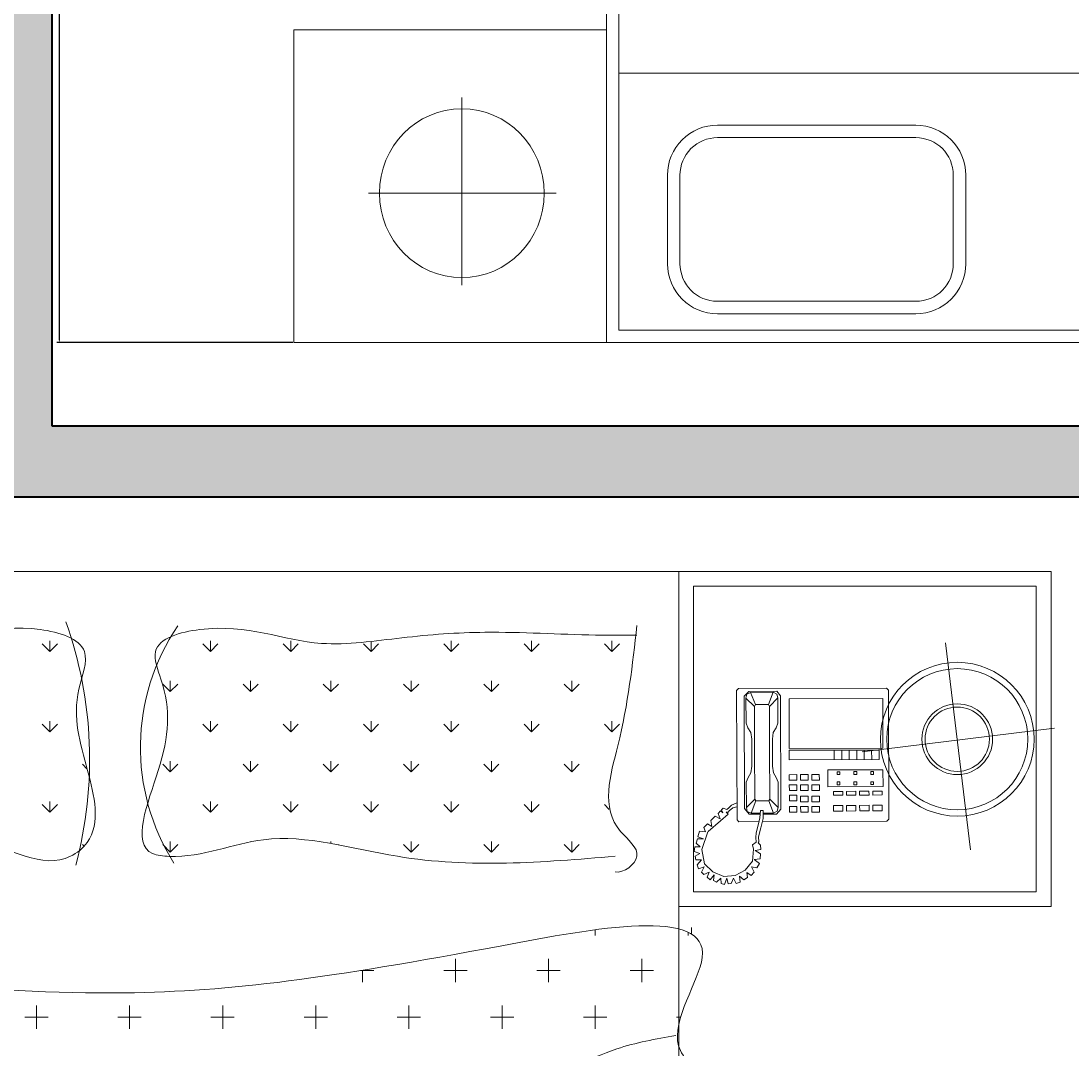
# Model space of a CAD drawing. Units: inches. Extents: x 2330 to 3943, y 1763 to 3461.
# Tile 20 of 40: x 3157 to 3231, y 2662 to 2734. Entities that reach past the tile are written whole.
import ezdxf

# ---------------------------------------------------------------- set-up
doc = ezdxf.new("R2010")
doc.units = ezdxf.units.IN
for name, color, linetype, lineweight in [('A-ANNO-DIMS', 2, 'Continuous', 18), ('A-FURN', 8, 'Continuous', 13), ('A-WALL', 7, 'Continuous', 40), ('A-WALL-PATT', 252, 'Continuous', 13)]:
    doc.layers.add(name, color=color, linetype=linetype, lineweight=lineweight)
doc.styles.get("Standard").update_dxf_attribs({"font": 'arial.ttf'})
doc.dimstyles.get("Standard").update_dxf_attribs({"dimtxt": 0.18, "dimasz": 0.18, "dimexe": 0.18, "dimexo": 0.0625, "dimgap": 0.09, "dimtad": 0, "dimtih": 1, "dimtoh": 1, "dimdec": 4, "dimzin": 0, "dimdsep": 46, "dimtxsty": 'Standard', "dimcen": 0.09, "dimadec": 0, "dimazin": 0, "dimtfac": 1, "dimtdec": 4, "dimtofl": 0, "dimtmove": 0, "dimatfit": 3, "dimfxl": 1, "dimtolj": 1, "dimtzin": 0, "dimarcsym": 0})

# ---------------------------------------------------------------- blocks, each defined once
blk = doc.blocks.new('A$C200C7901')
for p, q in [((0.5, 2.3334), (2, 2.3334)), ((2, 2.3334), (2.5, 2.3334)), ((2, 1.6055), (2, 2.3334)), ((2.5, 1.8834), (2.5, 2.3334)), ((1.3176, 2.1721), (1.3075, 2.1822)), ((1.3176, 2.1721), (1.3075, 2.1822)), ((1.206, 2.0681), (1.1997, 2.0744)), ((1.206, 2.0681), (1.1997, 2.0744)), ((1.2019, 1.9645), (1.1997, 1.9666)), ((1.2019, 1.9645), (1.1997, 1.9666)), ((2, 1.8834), (2.5, 1.8834)), ((2.0129, 1.8445), (2.0129, 1.849)), ((2.0129, 1.8445), (2.0129, 1.849)), ((2.0171, 1.8467), (2.0171, 1.8556)), ((2.0171, 1.8467), (2.0171, 1.8556)), ((1.1379, 1.7195), (1.1379, 1.7508)), ((1.1222, 1.7352), (1.1535, 1.7352)), ((1.9972, 1.7352), (2.0027, 1.7352)), ((1.9972, 1.7352), (2.0027, 1.7352)), ((2, 1.6963), (2, 1.7248)), ((2, 1.6963), (2, 1.7248))]:
    blk.add_line(p, q)
at = {"linetype": 'ByBlock'}
for p, q in [((2.02, 2.3134), (2.48, 2.3134)), ((2.02, 1.9034), (2.02, 2.3134)), ((2.48, 1.9034), (2.48, 2.3134)), ((1.1559, 2.2259), (1.1458, 2.236)), ((1.1559, 2.2259), (1.1458, 2.236)), ((1.1559, 2.2259), (1.1559, 2.2402)), ((1.1559, 2.2259), (1.1559, 2.2402)), ((1.1559, 2.2259), (1.166, 2.236)), ((1.1559, 2.2259), (1.166, 2.236)), ((1.3714, 2.2259), (1.3613, 2.236)), ((1.3714, 2.2259), (1.3613, 2.236)), ((1.3714, 2.2259), (1.3714, 2.2402)), ((1.3714, 2.2259), (1.3714, 2.2402)), ((1.3714, 2.2259), (1.3815, 2.236)), ((1.3714, 2.2259), (1.3815, 2.236)), ((1.4792, 2.2259), (1.4691, 2.236)), ((1.4792, 2.2259), (1.4691, 2.236)), ((1.4792, 2.2259), (1.4792, 2.2402)), ((1.4792, 2.2259), (1.4792, 2.2402)), ((1.4792, 2.2259), (1.4893, 2.236)), ((1.4792, 2.2259), (1.4893, 2.236)), ((1.587, 2.2259), (1.5769, 2.236)), ((1.587, 2.2259), (1.5769, 2.236)), ((1.587, 2.2259), (1.587, 2.2393)), ((1.587, 2.2259), (1.587, 2.2393)), ((1.587, 2.2259), (1.5971, 2.236)), ((1.587, 2.2259), (1.5971, 2.236)), ((1.6947, 2.2259), (1.6846, 2.236)), ((1.6947, 2.2259), (1.6846, 2.236)), ((1.6947, 2.2259), (1.6947, 2.2402)), ((1.6947, 2.2259), (1.6947, 2.2402)), ((1.6947, 2.2259), (1.7048, 2.236)), ((1.6947, 2.2259), (1.7048, 2.236)), ((1.8025, 2.2259), (1.7924, 2.236)), ((1.8025, 2.2259), (1.7924, 2.236)), ((1.8025, 2.2259), (1.8025, 2.2402)), ((1.8025, 2.2259), (1.8025, 2.2402)), ((1.8025, 2.2259), (1.8126, 2.236)), ((1.8025, 2.2259), (1.8126, 2.236)), ((1.9103, 2.2259), (1.9002, 2.236)), ((1.9103, 2.2259), (1.9002, 2.236)), ((1.9103, 2.2259), (1.9103, 2.2402)), ((1.9103, 2.2259), (1.9103, 2.2402)), ((1.9103, 2.2259), (1.9204, 2.236)), ((1.9103, 2.2259), (1.9204, 2.236)), ((2.3581, 2.2373), (2.3919, 1.9595)), ((1.3176, 2.172), (1.3176, 2.1863)), ((1.3176, 2.172), (1.3176, 2.1863)), ((1.4253, 2.172), (1.4253, 2.1863)), ((1.4253, 2.172), (1.4253, 2.1863)), ((1.5331, 2.172), (1.5331, 2.1863)), ((1.5331, 2.172), (1.5331, 2.1863)), ((1.6408, 2.172), (1.6408, 2.1863)), ((1.6408, 2.172), (1.6408, 2.1863)), ((1.7486, 2.172), (1.7486, 2.1863)), ((1.7486, 2.172), (1.7486, 2.1863)), ((1.8564, 2.172), (1.8564, 2.1863)), ((1.8564, 2.172), (1.8564, 2.1863)), ((1.3176, 2.1721), (1.3277, 2.1822)), ((1.3176, 2.1721), (1.3277, 2.1822)), ((1.4253, 2.1721), (1.4152, 2.1822)), ((1.4253, 2.1721), (1.4152, 2.1822)), ((1.4253, 2.1721), (1.4354, 2.1822)), ((1.4253, 2.1721), (1.4354, 2.1822)), ((1.5331, 2.1721), (1.523, 2.1822)), ((1.5331, 2.1721), (1.523, 2.1822)), ((1.5331, 2.1721), (1.5432, 2.1822)), ((1.5331, 2.1721), (1.5432, 2.1822)), ((1.6409, 2.1721), (1.6308, 2.1822)), ((1.6409, 2.1721), (1.6308, 2.1822)), ((1.6409, 2.1721), (1.651, 2.1822)), ((1.6409, 2.1721), (1.651, 2.1822)), ((1.7486, 2.1721), (1.7385, 2.1822)), ((1.7486, 2.1721), (1.7385, 2.1822)), ((1.7486, 2.1721), (1.7587, 2.1822)), ((1.7486, 2.1721), (1.7587, 2.1822)), ((1.8564, 2.1721), (1.8463, 2.1822)), ((1.8564, 2.1721), (1.8463, 2.1822)), ((1.8564, 2.1721), (1.8665, 2.1822)), ((1.8564, 2.1721), (1.8665, 2.1822)), ((2.0802, 2.176), (2.0777, 2.1734)), ((2.0777, 2.1734), (2.0783, 1.9999)), ((2.2789, 2.1766), (2.0802, 2.176)), ((2.0941, 2.1722), (2.0878, 2.1659)), ((2.0966, 2.171), (2.0915, 2.1685)), ((2.1318, 2.1724), (2.0941, 2.1722)), ((2.1267, 2.1711), (2.0966, 2.171)), ((2.1029, 2.1547), (2.0966, 2.171)), ((2.1205, 2.1547), (2.1267, 2.1711)), ((2.1267, 2.1711), (2.1318, 2.1686)), ((2.1368, 2.1661), (2.1318, 2.1724)), ((2.2789, 2.1766), (2.2814, 2.1741)), ((2.2814, 2.1741), (2.282, 2.0006)), ((2.0878, 2.1659), (2.0883, 2.015)), ((2.0915, 2.1685), (2.0903, 2.1634)), ((2.0903, 2.1634), (2.1017, 2.1521)), ((2.0903, 2.1634), (2.0904, 2.1295)), ((2.1331, 2.1636), (2.1218, 2.1522)), ((2.1318, 2.1686), (2.1331, 2.1636)), ((2.1331, 2.1636), (2.1332, 2.1296)), ((2.1373, 2.014), (2.1368, 2.1661)), ((2.1481, 2.1624), (2.2739, 2.1628)), ((2.1484, 2.0957), (2.1481, 2.1624)), ((2.2739, 2.1628), (2.2741, 2.0961)), ((2.1017, 2.1521), (2.1029, 2.1547)), ((2.1019, 2.0956), (2.1017, 2.1521)), ((2.1029, 2.1547), (2.1205, 2.1547)), ((2.1218, 2.1522), (2.1205, 2.1547)), ((2.122, 2.0956), (2.1218, 2.1522)), ((1.1559, 2.1182), (1.1458, 2.1283)), ((1.1559, 2.1182), (1.1458, 2.1283)), ((1.1559, 2.1182), (1.1559, 2.1325)), ((1.1559, 2.1182), (1.1559, 2.1325)), ((1.1559, 2.1182), (1.166, 2.1283)), ((1.1559, 2.1182), (1.166, 2.1283)), ((1.3714, 2.1182), (1.3613, 2.1283)), ((1.3714, 2.1182), (1.3613, 2.1283)), ((1.3714, 2.1182), (1.3714, 2.1325)), ((1.3714, 2.1182), (1.3714, 2.1325)), ((1.3714, 2.1182), (1.3815, 2.1283)), ((1.3714, 2.1182), (1.3815, 2.1283)), ((1.4792, 2.1182), (1.4691, 2.1283)), ((1.4792, 2.1182), (1.4691, 2.1283)), ((1.4792, 2.1182), (1.4792, 2.1325)), ((1.4792, 2.1182), (1.4792, 2.1325)), ((1.4792, 2.1182), (1.4893, 2.1283)), ((1.4792, 2.1182), (1.4893, 2.1283)), ((1.587, 2.1182), (1.5769, 2.1283)), ((1.587, 2.1182), (1.5769, 2.1283)), ((1.587, 2.1182), (1.587, 2.1325)), ((1.587, 2.1182), (1.587, 2.1325)), ((1.587, 2.1182), (1.5971, 2.1283)), ((1.587, 2.1182), (1.5971, 2.1283)), ((1.6947, 2.1182), (1.6846, 2.1283)), ((1.6947, 2.1182), (1.6846, 2.1283)), ((1.6947, 2.1182), (1.6947, 2.1325)), ((1.6947, 2.1182), (1.6947, 2.1325)), ((1.6947, 2.1182), (1.7048, 2.1283)), ((1.6947, 2.1182), (1.7048, 2.1283)), ((1.8025, 2.1182), (1.7924, 2.1283)), ((1.8025, 2.1182), (1.7924, 2.1283)), ((1.8025, 2.1182), (1.8025, 2.1325)), ((1.8025, 2.1182), (1.8025, 2.1325)), ((1.8025, 2.1182), (1.8126, 2.1283)), ((1.8025, 2.1182), (1.8126, 2.1283)), ((1.9103, 2.1182), (1.9002, 2.1283)), ((1.9103, 2.1182), (1.9002, 2.1283)), ((1.9103, 2.1182), (1.9103, 2.1325)), ((1.9103, 2.1182), (1.9103, 2.1325)), ((1.9103, 2.1182), (1.9204, 2.1283)), ((1.9103, 2.1182), (1.9204, 2.1283)), ((2.0904, 2.1295), (2.093, 2.1232)), ((2.1332, 2.1296), (2.1307, 2.1233)), ((2.093, 2.1232), (2.0968, 2.1169)), ((2.0968, 2.1169), (2.098, 2.1081)), ((2.1269, 2.117), (2.1257, 2.1082)), ((2.1307, 2.1233), (2.1269, 2.117)), ((2.2464, 2.0911), (2.5044, 2.1228)), ((2.098, 2.1081), (2.0981, 2.0956)), ((2.1257, 2.1082), (2.1257, 2.0956)), ((2.0982, 2.0717), (2.0981, 2.0956)), ((2.1019, 2.0956), (2.1021, 2.0277)), ((2.122, 2.0956), (2.1222, 2.0277)), ((2.1258, 2.0718), (2.1257, 2.0956)), ((2.2741, 2.0961), (2.1484, 2.0957)), ((2.1484, 2.0932), (2.2691, 2.0936)), ((2.1484, 2.0806), (2.1484, 2.0932)), ((2.2087, 2.0934), (2.2088, 2.0808)), ((2.2188, 2.0934), (2.2188, 2.0809)), ((2.2288, 2.0935), (2.2289, 2.0809)), ((2.2389, 2.0935), (2.239, 2.0809)), ((2.249, 2.0935), (2.249, 2.081)), ((2.259, 2.0936), (2.2591, 2.081)), ((2.2691, 2.0936), (2.2691, 2.081)), ((1.3176, 2.0643), (1.3075, 2.0744)), ((1.3176, 2.0643), (1.3075, 2.0744)), ((1.3176, 2.0643), (1.3176, 2.0786)), ((1.3176, 2.0643), (1.3176, 2.0786)), ((1.3176, 2.0643), (1.3277, 2.0744)), ((1.3176, 2.0643), (1.3277, 2.0744)), ((1.4253, 2.0643), (1.4152, 2.0744)), ((1.4253, 2.0643), (1.4152, 2.0744)), ((1.4253, 2.0643), (1.4253, 2.0786)), ((1.4253, 2.0643), (1.4253, 2.0786)), ((1.4253, 2.0643), (1.4354, 2.0744)), ((1.4253, 2.0643), (1.4354, 2.0744)), ((1.5331, 2.0643), (1.523, 2.0744)), ((1.5331, 2.0643), (1.523, 2.0744)), ((1.5331, 2.0643), (1.5331, 2.0786)), ((1.5331, 2.0643), (1.5331, 2.0786)), ((1.5331, 2.0643), (1.5432, 2.0744)), ((1.5331, 2.0643), (1.5432, 2.0744)), ((1.6409, 2.0643), (1.6308, 2.0744)), ((1.6409, 2.0643), (1.6308, 2.0744)), ((1.6408, 2.0643), (1.6408, 2.0786)), ((1.6408, 2.0643), (1.6408, 2.0786)), ((1.6409, 2.0643), (1.651, 2.0744)), ((1.6409, 2.0643), (1.651, 2.0744)), ((1.7486, 2.0643), (1.7385, 2.0744)), ((1.7486, 2.0643), (1.7385, 2.0744)), ((1.7486, 2.0643), (1.7486, 2.0786)), ((1.7486, 2.0643), (1.7486, 2.0786)), ((1.7486, 2.0643), (1.7587, 2.0744)), ((1.7486, 2.0643), (1.7587, 2.0744)), ((1.8564, 2.0643), (1.8463, 2.0744)), ((1.8564, 2.0643), (1.8463, 2.0744)), ((1.8564, 2.0643), (1.8564, 2.0786)), ((1.8564, 2.0643), (1.8564, 2.0786)), ((1.8564, 2.0643), (1.8665, 2.0744)), ((1.8564, 2.0643), (1.8665, 2.0744)), ((2.2691, 2.081), (2.1484, 2.0806)), ((2.0932, 2.0566), (2.0969, 2.0629)), ((2.0969, 2.0629), (2.0982, 2.0717)), ((2.1271, 2.063), (2.1258, 2.0718)), ((2.1309, 2.0567), (2.1271, 2.063)), ((2.1586, 2.0606), (2.1485, 2.0605)), ((2.1485, 2.0605), (2.1485, 2.053)), ((2.1586, 2.053), (2.1586, 2.0606)), ((2.1636, 2.0606), (2.1636, 2.053)), ((2.1736, 2.0606), (2.1636, 2.0606)), ((2.1737, 2.0531), (2.1736, 2.0606)), ((2.1887, 2.0607), (2.1787, 2.0606)), ((2.1787, 2.0606), (2.1787, 2.0531)), ((2.1888, 2.0531), (2.1887, 2.0607)), ((2.2, 2.067), (2.2742, 2.0672)), ((2.2001, 2.0443), (2.2, 2.067)), ((2.2126, 2.0645), (2.2164, 2.0645)), ((2.2126, 2.0607), (2.2126, 2.0645)), ((2.2164, 2.0607), (2.2126, 2.0607)), ((2.2164, 2.0645), (2.2164, 2.0607)), ((2.2352, 2.0646), (2.239, 2.0646)), ((2.2352, 2.0608), (2.2352, 2.0646)), ((2.239, 2.0608), (2.2352, 2.0608)), ((2.239, 2.0646), (2.239, 2.0608)), ((2.2579, 2.0609), (2.2579, 2.0647)), ((2.2579, 2.0647), (2.2616, 2.0647)), ((2.2616, 2.0609), (2.2579, 2.0609)), ((2.2616, 2.0647), (2.2616, 2.0609)), ((2.2742, 2.0672), (2.2743, 2.0446)), ((2.0907, 2.0503), (2.0932, 2.0566)), ((2.0908, 2.0163), (2.0907, 2.0503)), ((2.1334, 2.0504), (2.1309, 2.0567)), ((2.1336, 2.0165), (2.1334, 2.0504)), ((2.1485, 2.053), (2.1586, 2.053)), ((2.1485, 2.0467), (2.1486, 2.0391)), ((2.1586, 2.0467), (2.1485, 2.0467)), ((2.1586, 2.0392), (2.1586, 2.0467)), ((2.1636, 2.053), (2.1737, 2.0531)), ((2.1737, 2.0468), (2.1636, 2.0467)), ((2.1636, 2.0467), (2.1637, 2.0392)), ((2.1737, 2.0392), (2.1737, 2.0468)), ((2.1787, 2.0531), (2.1888, 2.0531)), ((2.1787, 2.0468), (2.1787, 2.0392)), ((2.1888, 2.0468), (2.1787, 2.0468)), ((2.1888, 2.0393), (2.1888, 2.0468)), ((2.2743, 2.0446), (2.2001, 2.0443)), ((2.2126, 2.0507), (2.2164, 2.0507)), ((2.2127, 2.0469), (2.2126, 2.0507)), ((2.2164, 2.0469), (2.2127, 2.0469)), ((2.2164, 2.0507), (2.2164, 2.0469)), ((2.2353, 2.0508), (2.2391, 2.0508)), ((2.2353, 2.047), (2.2353, 2.0508)), ((2.2391, 2.047), (2.2353, 2.047)), ((2.2391, 2.0508), (2.2391, 2.047)), ((2.2579, 2.0508), (2.2617, 2.0508)), ((2.2579, 2.0471), (2.2579, 2.0508)), ((2.2617, 2.0471), (2.2579, 2.0471)), ((2.2617, 2.0508), (2.2617, 2.0471)), ((2.1486, 2.0391), (2.1586, 2.0392)), ((2.1586, 2.0329), (2.1486, 2.0329)), ((2.1486, 2.0329), (2.1486, 2.0253)), ((2.1587, 2.0253), (2.1586, 2.0329)), ((2.1637, 2.0392), (2.1737, 2.0392)), ((2.1637, 2.0317), (2.1637, 2.0241)), ((2.1737, 2.0317), (2.1637, 2.0317)), ((2.1738, 2.0241), (2.1737, 2.0317)), ((2.1787, 2.0392), (2.1888, 2.0393)), ((2.1788, 2.0317), (2.1788, 2.0242)), ((2.1888, 2.0317), (2.1788, 2.0317)), ((2.1889, 2.0242), (2.1888, 2.0317)), ((2.2077, 2.0331), (2.2077, 2.0381)), ((2.2077, 2.0381), (2.2202, 2.0381)), ((2.2203, 2.0331), (2.2077, 2.0331)), ((2.2202, 2.0381), (2.2203, 2.0331)), ((2.2253, 2.0381), (2.2378, 2.0382)), ((2.2253, 2.0331), (2.2253, 2.0381)), ((2.2379, 2.0332), (2.2253, 2.0331)), ((2.2378, 2.0382), (2.2379, 2.0332)), ((2.2429, 2.0332), (2.2429, 2.0382)), ((2.2429, 2.0382), (2.2554, 2.0382)), ((2.2555, 2.0332), (2.2429, 2.0332)), ((2.2554, 2.0382), (2.2555, 2.0332)), ((2.2605, 2.0332), (2.2605, 2.0383)), ((2.2605, 2.0383), (2.273, 2.0383)), ((2.2731, 2.0333), (2.2605, 2.0332)), ((2.273, 2.0383), (2.2731, 2.0333)), ((1.1559, 2.0104), (1.1458, 2.0205)), ((1.1559, 2.0104), (1.1458, 2.0205)), ((1.1559, 2.0104), (1.1559, 2.0247)), ((1.1559, 2.0104), (1.1559, 2.0247)), ((1.1559, 2.0104), (1.166, 2.0205)), ((1.1559, 2.0104), (1.166, 2.0205)), ((1.3714, 2.0104), (1.3613, 2.0205)), ((1.3714, 2.0104), (1.3613, 2.0205)), ((1.3714, 2.0104), (1.3714, 2.0247)), ((1.3714, 2.0104), (1.3714, 2.0247)), ((1.3714, 2.0104), (1.3815, 2.0205)), ((1.3714, 2.0104), (1.3815, 2.0205)), ((1.4792, 2.0104), (1.4691, 2.0205)), ((1.4792, 2.0104), (1.4691, 2.0205)), ((1.4792, 2.0104), (1.4792, 2.0247)), ((1.4792, 2.0104), (1.4792, 2.0247)), ((1.4792, 2.0104), (1.4893, 2.0205)), ((1.4792, 2.0104), (1.4893, 2.0205)), ((1.587, 2.0104), (1.5769, 2.0205)), ((1.587, 2.0104), (1.5769, 2.0205)), ((1.587, 2.0104), (1.587, 2.0247)), ((1.587, 2.0104), (1.587, 2.0247)), ((1.587, 2.0104), (1.5971, 2.0205)), ((1.587, 2.0104), (1.5971, 2.0205)), ((1.6947, 2.0104), (1.6846, 2.0205)), ((1.6947, 2.0104), (1.6846, 2.0205)), ((1.6947, 2.0104), (1.6947, 2.0247)), ((1.6947, 2.0104), (1.6947, 2.0247)), ((1.6947, 2.0104), (1.7048, 2.0205)), ((1.6947, 2.0104), (1.7048, 2.0205)), ((1.8025, 2.0104), (1.7924, 2.0205)), ((1.8025, 2.0104), (1.7924, 2.0205)), ((1.8025, 2.0104), (1.8025, 2.0247)), ((1.8025, 2.0104), (1.8025, 2.0247)), ((1.8025, 2.0104), (1.8126, 2.0205)), ((1.8025, 2.0104), (1.8126, 2.0205)), ((1.9068, 2.0139), (1.9002, 2.0205)), ((1.9068, 2.0139), (1.9002, 2.0205)), ((2.0576, 2.0133), (2.0598, 2.0155)), ((2.0598, 2.0155), (2.0645, 2.0137)), ((2.0645, 2.0137), (2.0671, 2.0162)), ((2.0671, 2.0162), (2.0707, 2.0197)), ((2.0727, 2.016), (2.0676, 2.012)), ((2.0707, 2.0197), (2.0782, 2.0226)), ((2.0782, 2.0175), (2.0727, 2.016)), ((2.0908, 2.0163), (2.1021, 2.0277)), ((2.0921, 2.0113), (2.0908, 2.0163)), ((2.1034, 2.0252), (2.0971, 2.0088)), ((2.1021, 2.0277), (2.1034, 2.0252)), ((2.1034, 2.0252), (2.121, 2.0252)), ((2.1222, 2.0277), (2.121, 2.0252)), ((2.121, 2.0252), (2.1273, 2.0089)), ((2.1336, 2.0165), (2.1222, 2.0277)), ((2.1323, 2.0114), (2.1336, 2.0165)), ((2.1486, 2.0253), (2.1587, 2.0253)), ((2.1587, 2.0178), (2.1486, 2.0178)), ((2.1486, 2.0178), (2.1487, 2.0102)), ((2.1587, 2.0103), (2.1587, 2.0178)), ((2.1637, 2.0241), (2.1738, 2.0241)), ((2.1738, 2.0179), (2.1637, 2.0178)), ((2.1637, 2.0178), (2.1638, 2.0103)), ((2.1738, 2.0103), (2.1738, 2.0179)), ((2.1788, 2.0242), (2.1889, 2.0242)), ((2.1788, 2.0179), (2.1788, 2.0103)), ((2.1889, 2.0179), (2.1788, 2.0179)), ((2.1889, 2.0104), (2.1889, 2.0179)), ((2.2203, 2.0193), (2.2077, 2.0192)), ((2.2077, 2.0192), (2.2078, 2.0117)), ((2.2203, 2.0117), (2.2203, 2.0193)), ((2.2379, 2.0193), (2.2253, 2.0193)), ((2.2253, 2.0193), (2.2254, 2.0117)), ((2.2379, 2.0118), (2.2379, 2.0193)), ((2.2555, 2.0194), (2.2429, 2.0193)), ((2.2429, 2.0193), (2.243, 2.0118)), ((2.2555, 2.0118), (2.2555, 2.0194)), ((2.2605, 2.0194), (2.2606, 2.0119)), ((2.2731, 2.0194), (2.2605, 2.0194)), ((2.2731, 2.0119), (2.2731, 2.0194)), ((2.0431, 1.999), (2.0488, 2.0046)), ((2.0488, 2.0046), (2.0557, 2.0011)), ((2.053, 2.0084), (2.0563, 2.0119)), ((2.0557, 2.0011), (2.053, 2.0084)), ((2.0663, 2.0077), (2.0561, 1.9986)), ((2.0563, 2.0119), (2.0594, 2.0095)), ((2.0594, 2.0095), (2.0576, 2.0133)), ((2.0663, 2.0102), (2.0636, 2.0104)), ((2.0636, 2.0104), (2.0663, 2.0077)), ((2.0676, 2.012), (2.0663, 2.0102)), ((2.0883, 2.015), (2.0946, 2.0075)), ((2.0971, 2.0088), (2.0921, 2.0113)), ((2.0946, 2.0075), (2.1093, 2.0076)), ((2.1094, 2.0088), (2.0971, 2.0088)), ((2.1072, 1.9944), (2.109, 2.0025)), ((2.109, 2.0025), (2.1097, 2.0126)), ((2.1097, 2.0126), (2.1135, 2.0126)), ((2.1133, 2.0018), (2.1103, 1.989)), ((2.1135, 2.0126), (2.1133, 2.0018)), ((2.1273, 2.0089), (2.1134, 2.0088)), ((2.1134, 2.0076), (2.1311, 2.0077)), ((2.1273, 2.0089), (2.1323, 2.0114)), ((2.1311, 2.0077), (2.1373, 2.014)), ((2.1487, 2.0102), (2.1587, 2.0103)), ((2.1638, 2.0103), (2.1738, 2.0103)), ((2.1788, 2.0103), (2.1889, 2.0104)), ((2.2078, 2.0117), (2.2203, 2.0117)), ((2.2254, 2.0117), (2.2379, 2.0118)), ((2.243, 2.0118), (2.2555, 2.0118)), ((2.2606, 2.0119), (2.2731, 2.0119)), ((2.0338, 1.9895), (2.0386, 1.9946)), ((2.0358, 1.9839), (2.0338, 1.9895)), ((2.0386, 1.9946), (2.0444, 1.9911)), ((2.0561, 1.9986), (2.0396, 1.9844)), ((2.0444, 1.9911), (2.0431, 1.999)), ((2.0783, 1.9999), (2.0808, 1.9974)), ((2.0808, 1.9974), (2.1079, 1.9975)), ((2.1042, 1.9824), (2.1072, 1.9944)), ((2.1103, 1.989), (2.1073, 1.9771)), ((2.1123, 1.9975), (2.2795, 1.9981)), ((2.282, 2.0006), (2.2795, 1.9981)), ((2.0234, 1.9686), (2.0251, 1.9745)), ((2.0251, 1.9745), (2.0333, 1.9743)), ((2.0259, 1.977), (2.0281, 1.9847)), ((2.0333, 1.9743), (2.0259, 1.977)), ((2.0281, 1.9847), (2.0358, 1.9839)), ((2.0393, 1.984), (2.031, 1.96)), ((2.1035, 1.9763), (2.1042, 1.9824)), ((2.1038, 1.9697), (2.1035, 1.9763)), ((2.1073, 1.9771), (2.1076, 1.9704)), ((1.3176, 1.9565), (1.3075, 1.9666)), ((1.3176, 1.9565), (1.3075, 1.9666)), ((1.3176, 1.9565), (1.3176, 1.9708)), ((1.3176, 1.9565), (1.3176, 1.9708)), ((1.3176, 1.9565), (1.3277, 1.9666)), ((1.3176, 1.9565), (1.3277, 1.9666)), ((1.4253, 1.9703), (1.4253, 1.9708)), ((1.4253, 1.9703), (1.4253, 1.9708)), ((1.5331, 1.9683), (1.5331, 1.9708)), ((1.5331, 1.9683), (1.5331, 1.9708)), ((1.543, 1.9665), (1.5432, 1.9666)), ((1.543, 1.9665), (1.5432, 1.9666)), ((1.6409, 1.9565), (1.6308, 1.9666)), ((1.6409, 1.9565), (1.6308, 1.9666)), ((1.6408, 1.9565), (1.6408, 1.9708)), ((1.6408, 1.9565), (1.6408, 1.9708)), ((1.6409, 1.9565), (1.651, 1.9666)), ((1.6409, 1.9565), (1.651, 1.9666)), ((1.7486, 1.9565), (1.7385, 1.9666)), ((1.7486, 1.9565), (1.7385, 1.9666)), ((1.7486, 1.9565), (1.7486, 1.9708)), ((1.7486, 1.9565), (1.7486, 1.9708)), ((1.7486, 1.9565), (1.7587, 1.9666)), ((1.7486, 1.9565), (1.7587, 1.9666)), ((1.8564, 1.9565), (1.8463, 1.9666)), ((1.8564, 1.9565), (1.8463, 1.9666)), ((1.8564, 1.9565), (1.8564, 1.9708)), ((1.8564, 1.9565), (1.8564, 1.9708)), ((1.8564, 1.9565), (1.8665, 1.9666)), ((1.8564, 1.9565), (1.8665, 1.9666)), ((2.0206, 1.9572), (2.0218, 1.9635)), ((2.0218, 1.9635), (2.0287, 1.9636)), ((2.0287, 1.9636), (2.0234, 1.9686)), ((2.031, 1.96), (2.0346, 1.9409)), ((2.099, 1.9444), (2.1002, 1.9605)), ((2.0992, 1.9663), (2.1038, 1.9697)), ((2.1002, 1.9605), (2.0992, 1.9663)), ((2.1101, 1.96), (2.1028, 1.9587)), ((2.1076, 1.9704), (2.1068, 1.9689)), ((2.1068, 1.9689), (2.1096, 1.9661)), ((2.1096, 1.9661), (2.1101, 1.96)), ((2.0285, 1.9549), (2.0206, 1.9572)), ((2.0219, 1.9511), (2.0285, 1.9549)), ((2.0229, 1.946), (2.0219, 1.9511)), ((2.0308, 1.9462), (2.0229, 1.946)), ((2.0247, 1.9394), (2.0308, 1.9462)), ((2.1094, 1.9475), (2.1013, 1.9467)), ((2.1013, 1.9467), (2.1084, 1.9412)), ((2.1028, 1.9587), (2.1099, 1.9544)), ((2.1099, 1.9544), (2.1094, 1.9475)), ((2.0268, 1.9343), (2.0247, 1.9394)), ((2.0341, 1.9366), (2.0268, 1.9343)), ((2.0306, 1.9297), (2.0341, 1.9366)), ((2.0346, 1.9409), (2.0459, 1.93)), ((2.0759, 1.925), (2.0894, 1.9322)), ((2.0894, 1.9322), (2.099, 1.9444)), ((2.1051, 1.9353), (2.0975, 1.9368)), ((2.0975, 1.9368), (2.1011, 1.9297)), ((2.1084, 1.9412), (2.1051, 1.9353)), ((2.0339, 1.9267), (2.0306, 1.9297)), ((2.041, 1.9297), (2.0339, 1.9267)), ((2.038, 1.9228), (2.041, 1.9297)), ((2.0421, 1.9193), (2.038, 1.9228)), ((2.0474, 1.9259), (2.0421, 1.9193)), ((2.0459, 1.93), (2.0607, 1.9237)), ((2.0467, 1.9183), (2.0474, 1.9259)), ((2.0508, 1.9163), (2.0467, 1.9183)), ((2.0566, 1.9214), (2.0508, 1.9163)), ((2.0569, 1.9145), (2.0566, 1.9214)), ((2.0607, 1.9237), (2.0759, 1.925)), ((2.0645, 1.9214), (2.0617, 1.9133)), ((2.0663, 1.914), (2.0645, 1.9214)), ((2.0736, 1.9214), (2.0706, 1.9146)), ((2.077, 1.9146), (2.0736, 1.9214)), ((2.0876, 1.9195), (2.0815, 1.9245)), ((2.0815, 1.9245), (2.0823, 1.9161)), ((2.0925, 1.9225), (2.0876, 1.9195)), ((2.0973, 1.9251), (2.0914, 1.9294)), ((2.0914, 1.9294), (2.0925, 1.9225)), ((2.1011, 1.9297), (2.0973, 1.9251)), ((2.02, 1.9034), (2.48, 1.9034)), ((2.0617, 1.9133), (2.0569, 1.9145)), ((2.0706, 1.9146), (2.0663, 1.914)), ((2.0823, 1.9161), (2.077, 1.9146)), ((1.8879, 1.8445), (1.8879, 1.8523)), ((1.8879, 1.8445), (1.8879, 1.8523)), ((1.7004, 1.782), (1.7004, 1.8133)), ((1.7004, 1.782), (1.7004, 1.8133)), ((1.8254, 1.782), (1.8254, 1.8133)), ((1.8254, 1.782), (1.8254, 1.8133)), ((1.9504, 1.782), (1.9504, 1.8133)), ((1.9504, 1.782), (1.9504, 1.8133)), ((1.573, 1.7977), (1.591, 1.7977)), ((1.573, 1.7977), (1.591, 1.7977)), ((1.5754, 1.782), (1.5754, 1.7981)), ((1.5754, 1.782), (1.5754, 1.7981)), ((1.6847, 1.7977), (1.716, 1.7977)), ((1.6847, 1.7977), (1.716, 1.7977)), ((1.8097, 1.7977), (1.841, 1.7977)), ((1.8097, 1.7977), (1.841, 1.7977)), ((1.9347, 1.7977), (1.966, 1.7977)), ((1.9347, 1.7977), (1.966, 1.7977)), ((1.1379, 1.7195), (1.1379, 1.7508)), ((1.2629, 1.7195), (1.2629, 1.7508)), ((1.2629, 1.7195), (1.2629, 1.7508)), ((1.3879, 1.7195), (1.3879, 1.7508)), ((1.3879, 1.7195), (1.3879, 1.7508)), ((1.5129, 1.7195), (1.5129, 1.7508)), ((1.5129, 1.7195), (1.5129, 1.7508)), ((1.6379, 1.7195), (1.6379, 1.7508)), ((1.6379, 1.7195), (1.6379, 1.7508)), ((1.7629, 1.7195), (1.7629, 1.7508)), ((1.7629, 1.7195), (1.7629, 1.7508)), ((1.8879, 1.7195), (1.8879, 1.7508)), ((1.8879, 1.7195), (1.8879, 1.7508)), ((1.1222, 1.7352), (1.1535, 1.7352)), ((1.2472, 1.7352), (1.2785, 1.7352)), ((1.2472, 1.7352), (1.2785, 1.7352)), ((1.3722, 1.7352), (1.4035, 1.7352)), ((1.3722, 1.7352), (1.4035, 1.7352)), ((1.4972, 1.7352), (1.5285, 1.7352)), ((1.4972, 1.7352), (1.5285, 1.7352)), ((1.6222, 1.7352), (1.6535, 1.7352)), ((1.6222, 1.7352), (1.6535, 1.7352)), ((1.7472, 1.7352), (1.7785, 1.7352)), ((1.7472, 1.7352), (1.7785, 1.7352)), ((1.8722, 1.7352), (1.9035, 1.7352)), ((1.8722, 1.7352), (1.9035, 1.7352))]:
    blk.add_line(p, q, dxfattribs=at)
for radius in [0.1032, 0.0947, 0.0475, 0.0432]:
    blk.add_circle((2.3739, 2.1081), radius, dxfattribs=at)
for centre, radius, start, end in [((0.658, 2.0811), 0.5513, 345.0722, 19.5492), ((1.5685, 2.097), 0.291, 145.8603, 212.2445)]:
    blk.add_arc(centre, radius, start, end)
for points, knots in [([(0.5854, 1.951), (0.6835, 1.9407), (0.8425, 1.9242), (1.0374, 2.0054), (1.1564, 1.9255), (1.2274, 1.9841), (1.2052, 2.0751), (1.1815, 2.152), (1.2176, 2.2368), (1.0992, 2.2731), (1.0008, 2.2255), (0.8698, 2.246), (0.7481, 2.2548), (0.6426, 2.2473), (0.5746, 2.2478), (0.5562, 2.2479)], [0, 0, 0, 0, 292.165466, 473.33038, 601.631673, 630.723769, 727.138505, 836.819956, 887.958136, 954.42438, 1118.989809, 1227.016542, 1338.750986, 1487.447361, 1542.751028, 1542.751028, 1542.751028, 1542.751028]), ([(1.9146, 1.951), (1.8174, 1.9428), (1.6601, 1.9297), (1.4574, 1.9942), (1.3549, 1.9462), (1.2593, 1.9563), (1.314, 2.0834), (1.3193, 2.1569), (1.2853, 2.2393), (1.4031, 2.2724), (1.4987, 2.2256), (1.6304, 2.2459), (1.7519, 2.2548), (1.8574, 2.2473), (1.9254, 2.2478), (1.9438, 2.2479)], [0, 0, 0, 0, 292.165466, 473.33038, 601.631673, 624.236147, 735.870502, 858.452188, 896.317728, 962.783971, 1127.3494, 1235.376134, 1347.110578, 1495.806953, 1551.11062, 1551.11062, 1551.11062, 1551.11062]), ([(1.9438, 2.2608), (1.9381, 2.2086), (1.9282, 2.1195), (1.8897, 2.0022), (1.9591, 1.9538), (1.9264, 1.9278), (1.9146, 1.93)], [0, 0, 0, 0, 163.411291, 278.570782, 318.445997, 354.484131, 354.484131, 354.484131, 354.484131]), ([(0.4485, 1.7835), (0.4321, 1.7496), (0.4062, 1.6964), (0.49, 1.6713), (0.4719, 1.5969), (0.4123, 1.592), (0.4233, 1.5337), (0.4954, 1.5086), (0.4012, 1.4738), (0.3253, 1.4306), (0.4113, 1.3764), (0.3688, 1.3065), (0.5579, 1.2663), (0.741, 1.4533), (1.1127, 1.1109), (1.4811, 1.2478), (1.7885, 1.3492), (2.0357, 1.1637), (2.0748, 1.2974), (2.0876, 1.349), (2.0192, 1.3805), (2.0564, 1.4298), (2.0588, 1.4846), (1.9759, 1.5349), (2.1004, 1.5845), (2.0397, 1.6519), (1.971, 1.7053), (2.1104, 1.8981), (1.5946, 1.7967), (1.2448, 1.7472), (0.8129, 1.7935), (0.4953, 1.8548), (0.4582, 1.7983), (0.4485, 1.7835)], [0, 0, 0, 0, 88.420092, 139.08588, 204.302936, 239.695496, 287.801042, 327.365471, 412.960499, 463.626286, 552.059846, 584.668336, 662.614915, 940.993281, 1309.926334, 1844.022653, 1996.276242, 2316.43048, 2341.441004, 2404.707416, 2449.463774, 2514.680778, 2538.40571, 2613.031547, 2697.13096, 2760.903931, 2822.692699, 2945.47, 3215.060018, 3725.584917, 4361.974444, 4504.671998, 4555.32777, 4555.32777, 4555.32777, 4555.32777])]:
    blk.add_open_spline(points, degree=3, knots=knots)
blk.add_open_spline([(1.996, 1.7104), (1.9692, 1.7057), (1.9025, 1.6938), (1.844, 1.6592), (1.809, 1.6385)], degree=3, knots=[0, 0, 0, 0, 81.132613, 201.738644, 201.738644, 201.738644, 201.738644], dxfattribs=at)
blk.add_open_spline([(1.996, 1.7104), (1.9692, 1.7057), (1.9025, 1.6938), (1.844, 1.6592), (1.809, 1.6385)], degree=3, knots=[0, 0, 0, 0, 81.132613, 201.738644, 201.738644, 201.738644, 201.738644], dxfattribs=at)
blk = doc.blocks.new('A$C057D194F')
for p, q in [((2, 2, -0.1688), (0.5, 2, -0.1688)), ((2, 0, -0.1688), (2, 2, -0.1688)), ((2.5, 2, -0.1688), (2, 2, -0.1688)), ((2.5, 1.5, -0.1688), (2.5, 2, -0.1688)), ((1.98, 1.98, -0.1688), (0.52, 1.98, -0.1688)), ((1.98, 0.02, -0.1688), (1.98, 1.98, -0.1688)), ((1.8224, 1.9539, -0.1688), (1.5052, 1.9539, -0.1688)), ((1.8224, 1.9339, -0.1688), (1.5052, 1.9339, -0.1688)), ((2.2313, 1.9081, -0.1688), (2.2313, 1.761, -0.1688)), ((2.2313, 1.6081, -0.1688), (2.2313, 1.9081, -0.1688)), ((1.4252, 1.8739, -0.1688), (1.4252, 1.7322, -0.1688)), ((1.4452, 1.8739, -0.1688), (1.4452, 1.7322, -0.1688)), ((1.8824, 1.7322, -0.1688), (1.8824, 1.8739, -0.1688)), ((1.9024, 1.7322, -0.1688), (1.9024, 1.8739, -0.1688)), ((2.0806, 1.761, -0.1688), (2.3806, 1.761, -0.1688)), ((2.2313, 1.761, -0.1688), (2.0806, 1.761, -0.1688)), ((2.2313, 1.761, -0.1688), (2.2313, 1.6081, -0.1688)), ((1.5052, 1.6722, -0.1688), (1.8224, 1.6722, -0.1688)), ((1.5052, 1.6522, -0.1688), (1.8224, 1.6522, -0.1688)), ((1.98, 1.5693, -0.1688), (0.52, 1.5693, -0.1688)), ((2, 1.5, -0.1688), (2.5, 1.5, -0.1688))]:
    blk.add_line(p, q)
for centre, radius, start, end in [((1.5052, 1.8739, -0.1688), 0.08, 90, 180), ((1.8224, 1.8739, -0.1688), 0.08, 0, 90), ((1.5052, 1.8739, -0.1688), 0.06, 90, 180), ((1.8224, 1.8739, -0.1688), 0.06, 0, 90), ((1.5052, 1.7322, -0.1688), 0.08, 180, 270), ((1.5052, 1.7322, -0.1688), 0.06, 180, 270), ((1.8224, 1.7322, -0.1688), 0.08, 270, 0), ((1.8224, 1.7322, -0.1688), 0.06, 270, 0)]:
    blk.add_arc(centre, radius, start, end)
at = {"extrusion": (0, 0, -1)}
blk.add_ellipse((2.2313, 1.761, -0.1688), major_axis=(0, 0.1351), ratio=0.975448, dxfattribs=at)
blk.add_point((2.2313, 1.761, -0.1688))
blk = doc.blocks.new('*D58')
at = {"layer": 'A-ANNO-DIMS', "color": 0, "lineweight": -2, "transparency": 16777216}
for p, q in [((3176.65, 2799.677), (3160.004, 2799.677)), ((3160.184, 2799.497), (3160.184, 2755.784)), ((3160.184, 2711.709), (3160.184, 2755.421)), ((3176.65, 2711.529), (3160.004, 2711.529))]:
    blk.add_line(p, q, dxfattribs=at)
at = {"layer": 'A-ANNO-DIMS', "color": 0, "transparency": 16777216}
for points in [[(3160.154, 2799.497), (3160.214, 2799.497), (3160.184, 2799.677)], [(3160.154, 2711.709), (3160.214, 2711.709), (3160.184, 2711.529)]]:
    blk.add_solid(points, dxfattribs=at)
at = {"layer": 'Defpoints', "color": 0, "transparency": 16777216}
for p in [(3176.712, 2799.677), (3160.184, 2711.529), (3176.712, 2711.529)]:
    blk.add_point(p, dxfattribs=at)
at = {"layer": 'A-ANNO-DIMS', "color": 0, "transparency": 16777216, "insert": (3160.184, 2755.603), "char_height": 0.18, "attachment_point": 5}
blk.add_mtext('\\A1;88', dxfattribs=at)
blk = doc.blocks.new('*D95')
at = {"layer": 'A-ANNO-DIMS', "color": 0, "lineweight": -2, "transparency": 16777216}
for p, q in [((3105.603, 2727.687), (3105.783, 2727.687)), ((3105.693, 2727.597), (3105.693, 2727.777)), ((3606.312, 2659.69), (3418.758, 2685.165))]:
    blk.add_line(p, q, dxfattribs=at)
at = {"layer": 'A-ANNO-DIMS', "color": 0, "transparency": 16777216}
blk.add_solid([(3418.762, 2685.195), (3418.754, 2685.135), (3418.58, 2685.189)], dxfattribs=at)
at = {"layer": 'Defpoints', "color": 0, "transparency": 16777216}
for p in [(3105.693, 2727.687), (3418.58, 2685.189)]:
    blk.add_point(p, dxfattribs=at)
at = {"layer": 'A-ANNO-DIMS', "color": 0, "transparency": 16777216, "insert": (3606.862, 2659.69), "char_height": 0.18, "attachment_point": 5}
blk.add_mtext('\\A1;R315.76', dxfattribs=at)
blk = doc.blocks.new('*D96')
at = {"layer": 'A-ANNO-DIMS', "color": 0, "lineweight": -2, "transparency": 16777216}
for p, q in [((3604.649, 2753.345), (3417.721, 2743.732)), ((3105.603, 2727.687), (3105.783, 2727.687)), ((3105.693, 2727.597), (3105.693, 2727.777))]:
    blk.add_line(p, q, dxfattribs=at)
at = {"layer": 'A-ANNO-DIMS', "color": 0, "transparency": 16777216}
blk.add_solid([(3417.719, 2743.762), (3417.722, 2743.702), (3417.541, 2743.723)], dxfattribs=at)
at = {"layer": 'Defpoints', "color": 0, "transparency": 16777216}
for p in [(3417.541, 2743.723), (3105.693, 2727.687)]:
    blk.add_point(p, dxfattribs=at)
at = {"layer": 'A-ANNO-DIMS', "color": 0, "transparency": 16777216, "insert": (3605.394, 2753.345), "char_height": 0.18, "attachment_point": 5}
blk.add_mtext('\\A1;2X R312.26', dxfattribs=at)
blk = doc.blocks.new('*D97')
at = {"layer": 'A-ANNO-DIMS', "color": 0, "lineweight": -2, "transparency": 16777216}
for p, q in [((3105.603, 2727.687), (3105.783, 2727.687)), ((3105.693, 2727.597), (3105.693, 2727.777)), ((3589.166, 2615.071), (3408.039, 2657.261))]:
    blk.add_line(p, q, dxfattribs=at)
at = {"layer": 'A-ANNO-DIMS', "color": 0, "transparency": 16777216}
blk.add_solid([(3408.046, 2657.29), (3408.032, 2657.232), (3407.864, 2657.302)], dxfattribs=at)
at = {"layer": 'Defpoints', "color": 0, "transparency": 16777216}
for p in [(3105.693, 2727.687), (3407.864, 2657.302)]:
    blk.add_point(p, dxfattribs=at)
at = {"layer": 'A-ANNO-DIMS', "color": 0, "transparency": 16777216, "insert": (3589.911, 2615.071), "char_height": 0.18, "attachment_point": 5}
blk.add_mtext('\\A1;2X R310.26', dxfattribs=at)
blk = doc.blocks.new('*D98')
at = {"layer": 'A-ANNO-DIMS', "color": 0, "lineweight": -2, "transparency": 16777216}
for p, q in [((3105.603, 2727.687), (3105.783, 2727.687)), ((3105.693, 2727.597), (3105.693, 2727.777)), ((3519.334, 2463.489), (3364.371, 2562.466)), ((3519.514, 2463.489), (3519.334, 2463.489))]:
    blk.add_line(p, q, dxfattribs=at)
at = {"layer": 'A-ANNO-DIMS', "color": 0, "transparency": 16777216}
blk.add_solid([(3364.387, 2562.491), (3364.355, 2562.441), (3364.219, 2562.563)], dxfattribs=at)
at = {"layer": 'Defpoints', "color": 0, "transparency": 16777216}
for p in [(3105.693, 2727.687), (3364.219, 2562.563)]:
    blk.add_point(p, dxfattribs=at)
at = {"layer": 'A-ANNO-DIMS', "color": 0, "transparency": 16777216, "insert": (3520.257, 2463.489), "char_height": 0.18, "attachment_point": 5}
blk.add_mtext('\\A1;3X R306.76', dxfattribs=at)

msp = doc.modelspace()

# ---------------------------------------------------------------- hatches: boundary and pattern name
at = {"layer": 'A-WALL-PATT'}
h = msp.add_hatch(color=256, dxfattribs=at)
h.dxf.hatch_style = 1
h.paths.add_polyline_path([(3420.6832, 2705.6524), (3159.6605, 2705.6524), (3159.6605, 2827.6524), (3154.6605, 2827.6524), (3154.6605, 2705.6524), (3017.6605, 2705.6524), (3017.6605, 2700.6524), (3238.6605, 2700.6524), (3238.6605, 2605.6524), (3247.6605, 2605.6524), (3247.6605, 2610.6524), (3243.6605, 2610.6524), (3243.6605, 2700.6524), (3411.2593, 2700.6524, -0.0252833), (3406.9698, 2669.9468), (3415.809, 2668.2528, 0.029888)])

# ---------------------------------------------------------------- linework, layer by layer
at = {"layer": 'A-WALL'}
for p, q in [((3159.6605, 2827.6524), (3159.6605, 2705.6524)), ((3159.6605, 2705.6524), (3420.6832, 2705.6524)), ((3017.6605, 2700.6524), (3238.6605, 2700.6524))]:
    msp.add_line(p, q, dxfattribs=at)

# ---------------------------------------------------------------- block references
at = {"layer": 'A-FURN', "xscale": 44.07393684478161, "yscale": 44.07393684478161, "zscale": 44.07393684478161, "rotation": 180}
msp.add_blockref('A$C057D194F', (3286.8969, 2799.6765, 7.4375), dxfattribs=at)
at = {"layer": 'A-FURN', "xscale": 52.5181391560459, "yscale": 52.5181391560459, "zscale": 52.5181391560459}
msp.add_blockref('A$C200C7901', (3098.8053, 2572.8601), dxfattribs=at)

# ---------------------------------------------------------------- dimensions: what is measured, and where the dimension line sits
at = {"layer": 'A-ANNO-DIMS'}
dim = msp.add_linear_dim(base=(3160.1844, 2711.5286), p1=(3176.7121, 2799.6765), p2=(3176.7121, 2711.5286), angle=270, dimstyle='Standard', override={"dimdec": 0, "dimlfac": 1, "dimrnd": 0, "dimzin": 0, "dimdsep": 46, "dimlunit": 2}, dxfattribs=at)
dim.commit()
dim.dimension.update_dxf_attribs({"geometry": '*D58', "text_midpoint": (3160.1844, 2755.6026)})
for mpoint, text, picture, middle in [((3417.5409, 2743.723), '2X <>', '*D96', (3604.6494, 2753.3446)), ((3407.8638, 2657.302), '2X <>', '*D97', (3589.166, 2615.0711)), ((3364.219, 2562.563), '3X <>', '*D98', (3520.2574, 2463.4886))]:
    dim = msp.add_radius_dim(center=(3105.6935, 2727.6869), mpoint=mpoint, text=text, dimstyle='Standard', override={"dimdec": 2, "dimlfac": 1, "dimrnd": 0, "dimzin": 0, "dimdsep": 46, "dimlunit": 2}, dxfattribs=at)
    dim.commit()
    dim.dimension.update_dxf_attribs({"geometry": picture, "text_midpoint": middle, "dimtype": 164})
dim = msp.add_radius_dim(center=(3105.6935, 2727.6869), mpoint=(3418.58, 2685.189), dimstyle='Standard', override={"dimdec": 2, "dimlfac": 1, "dimrnd": 0, "dimzin": 0, "dimdsep": 46, "dimlunit": 2}, dxfattribs=at)
dim.commit()
dim.dimension.update_dxf_attribs({"geometry": '*D95', "text_midpoint": (3606.3119, 2659.6902), "dimtype": 164})

doc.saveas('drawing.dxf')
